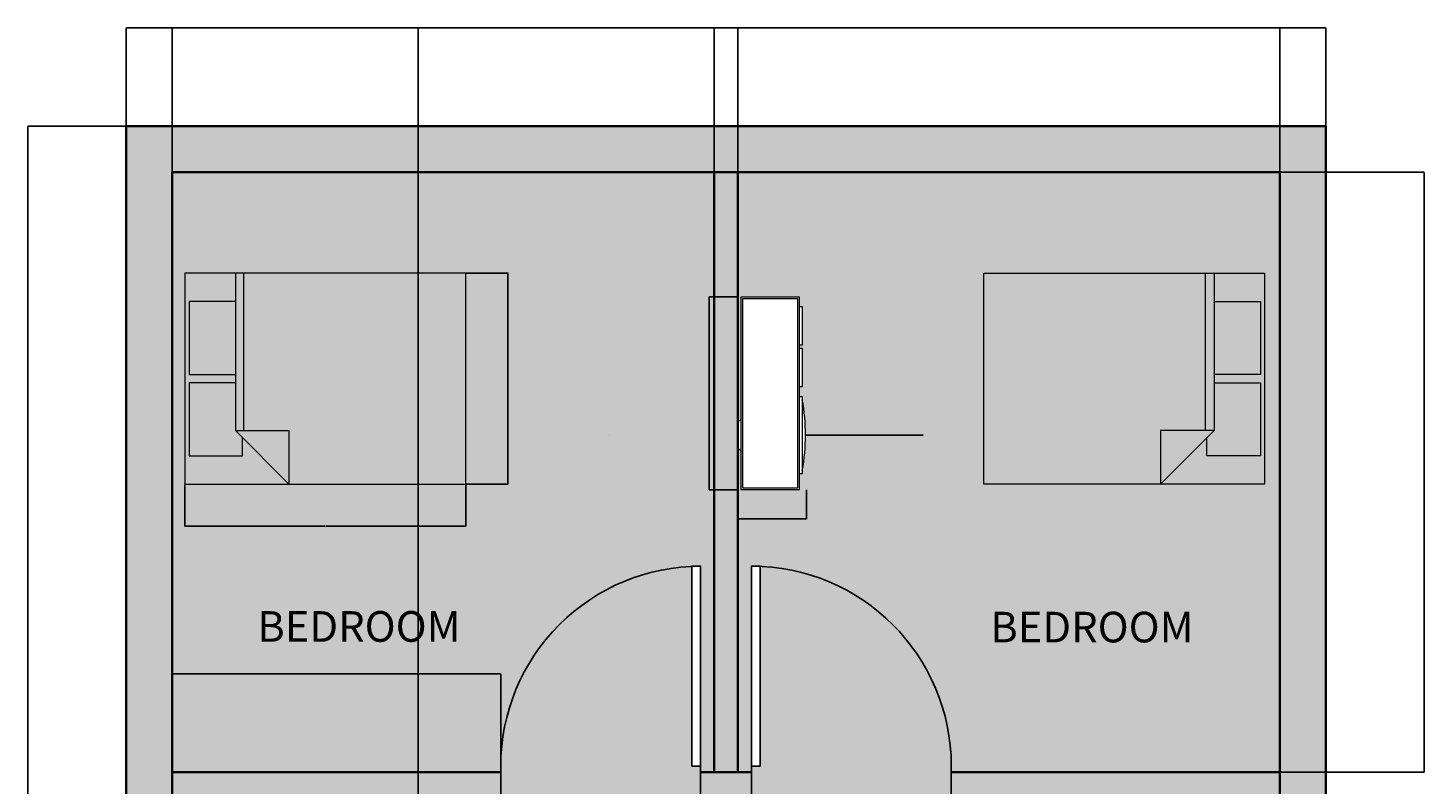
# Model space of a CAD drawing. Units: millimetres. Extents: x 1166 to 16630, y -7192 to 2820.
# Tile 8 of 8: x 9646 to 16630, y -963 to 2820. Entities that reach past the tile are written whole.
import ezdxf

# ---------------------------------------------------------------- set-up
doc = ezdxf.new("R2010")
doc.units = ezdxf.units.MM
for name, color, linetype, lineweight in [('A-ANNO-DIMS', 2, 'Continuous', 18), ('A-AREA-IDEN', 7, 'Continuous', 18), ('A-DOOR', 4, 'Continuous', 25), ('A-FURN', 8, 'Continuous', 18), ('A-WALL', 7, 'Continuous', 35)]:
    doc.layers.add(name, color=color, linetype=linetype, lineweight=lineweight)
for name, color, linetype, lineweight, true_color in [('A-FLOR-FNSH-PATT', 254, 'Continuous', 13, 0xfeeab9), ('A-FURN-PATT', 254, 'Continuous', 13, 0xd7c8d7), ('A-WALL-PATT', 254, 'Continuous', 13, 0xcecce6)]:
    doc.layers.add(name, color=color, linetype=linetype, lineweight=lineweight, true_color=true_color)
doc.styles.get("Standard").update_dxf_attribs({"font": 'arial.ttf'})
doc.dimstyles.get("Standard").update_dxf_attribs({"dimtxt": 0.18, "dimasz": 0.18, "dimexe": 0.18, "dimexo": 0.0625, "dimgap": 0.09, "dimtad": 0, "dimtih": 1, "dimtoh": 1, "dimdec": 4, "dimzin": 0, "dimdsep": 46, "dimtxsty": 'Standard', "dimcen": 0.09, "dimadec": 0, "dimazin": 0, "dimtfac": 1, "dimtdec": 4, "dimtofl": 0, "dimtmove": 0, "dimatfit": 3, "dimfxl": 1, "dimtolj": 1, "dimtzin": 0, "dimarcsym": 0})

# ---------------------------------------------------------------- blocks, each defined once
blk = doc.blocks.new('*U2')
for p, q in [((0, 0), (0, 6)), ((40, 0), (40, 6))]:
    blk.add_line(p, q)
blk.add_lwpolyline([(0, 0), (0, -40), (1.75, -40), (1.75, 0)], close=True)
blk.add_arc((0, 0), 40, 270, 0)
blk = doc.blocks.new('Bed - Queen')
for p, q in [((0, -80.00003), (0, 0)), ((0, 0), (59.99999, 0)), ((59.99999, 0), (59.99999, -80.00003)), ((7.99999, -1.2), (28.79998, -1.2)), ((7.99999, -14.4), (7.99999, -1.2)), ((28.79998, -1.2), (28.79998, -14.4)), ((31.19999, -1.2), (51.99999, -1.2)), ((31.19999, -14.4), (31.19999, -1.2)), ((51.99999, -1.2), (51.99999, -16.4)), ((0, -14.4), (44.8, -14.4)), ((59.99999, -29.6), (44.8, -14.4)), ((44.8, -14.4), (44.8, -29.6)), ((44.8, -16.8), (0, -16.8)), ((51.99999, -16.4), (46.79936, -16.4)), ((44.8, -29.6), (59.99999, -29.6)), ((59.99999, -80.00003), (0, -80.00003))]:
    blk.add_line(p, q)
blk = doc.blocks.new('Entertainment Center')
for p, q in [((-4, 0), (-5, -1)), ((4, 0), (-4, 0)), ((5, -1), (4, 0)), ((-17, -19), (-17, -1)), ((-17, -1), (43, -1)), ((-16.5, -18.5), (-16.5, -1.5)), ((-16.5, -1.5), (42.5, -1.5)), ((42.5, -1.5), (42.5, -18.5)), ((43, -1), (43, -19)), ((43, -19), (-17, -19)), ((42.5, -18.5), (-16.5, -18.5)), ((-12, -20), (-12, -19)), ((12, -20), (-12, -20)), ((12, -19), (12, -20)), ((15, -20), (15, -19)), ((27, -20), (15, -20)), ((27, -19), (27, -20)), ((28, -20), (28, -19)), ((40, -20), (28, -20)), ((40, -19), (40, -20))]:
    blk.add_line(p, q)
blk.add_arc((0, 40), 61, 259.6111, 280.3889)
blk = doc.blocks.new('*D15')
at = {"layer": 'A-ANNO-DIMS', "color": 0, "lineweight": -2, "transparency": 16777216}
for p, q in [((10431.5, 538.3), (10431.5, 327.4)), ((11836.7, 538.3), (11836.7, 327.4)), ((10431.7, 327.6), (11132.7, 327.6)), ((11836.6, 327.6), (11135.6, 327.6))]:
    blk.add_line(p, q, dxfattribs=at)
at = {"layer": 'A-ANNO-DIMS', "color": 0, "transparency": 16777216}
for points in [[(10431.7, 327.6), (10431.7, 327.5), (10431.5, 327.6)], [(11836.6, 327.6), (11836.6, 327.5), (11836.7, 327.6)]]:
    blk.add_solid(points, dxfattribs=at)
at = {"layer": 'Defpoints', "color": 0, "transparency": 16777216}
for p in [(10431.5, 538.4), (11836.7, 538.4), (10431.5, 327.6)]:
    blk.add_point(p, dxfattribs=at)
at = {"layer": 'A-ANNO-DIMS', "color": 0, "transparency": 16777216, "insert": (11134.1, 327.6), "char_height": 0.18, "attachment_point": 5}
blk.add_mtext('\\A1;QUEEN BED 1405 TYP.', dxfattribs=at)
blk = doc.blocks.new('*D16')
at = {"layer": 'A-ANNO-DIMS', "color": 0, "lineweight": -2, "transparency": 16777216}
for p, q in [((11836.8, 1592.3), (12047.7, 1592.3)), ((12047.5, 1592.1), (12047.5, 1065.5)), ((12047.5, 538.5), (12047.5, 1065.1)), ((11836.8, 538.4), (12047.7, 538.4))]:
    blk.add_line(p, q, dxfattribs=at)
at = {"layer": 'A-ANNO-DIMS', "color": 0, "transparency": 16777216}
for points in [[(12047.5, 1592.1), (12047.6, 1592.1), (12047.5, 1592.3)], [(12047.5, 538.5), (12047.6, 538.5), (12047.5, 538.4)]]:
    blk.add_solid(points, dxfattribs=at)
at = {"layer": 'Defpoints', "color": 0, "transparency": 16777216}
for p in [(11836.7, 1592.3), (11836.7, 538.4), (12047.5, 538.4)]:
    blk.add_point(p, dxfattribs=at)
at = {"layer": 'A-ANNO-DIMS', "color": 0, "transparency": 16777216, "insert": (12047.5, 1065.3), "char_height": 0.18, "attachment_point": 5}
blk.add_mtext('\\A1;1054 TYP.', dxfattribs=at)
blk = doc.blocks.new('*D19')
at = {"layer": 'A-ANNO-DIMS', "color": 0, "lineweight": -2, "transparency": 16777216}
for p, q in [((13198.1, 1474.7), (13053.2, 1474.7)), ((13053.4, 1474.5), (13053.4, 992.3)), ((13053.4, 509.7), (13053.4, 991.9)), ((13198.1, 509.5), (13053.2, 509.5))]:
    blk.add_line(p, q, dxfattribs=at)
at = {"layer": 'A-ANNO-DIMS', "color": 0, "transparency": 16777216}
for points in [[(13053.4, 1474.5), (13053.5, 1474.5), (13053.4, 1474.7)], [(13053.4, 509.7), (13053.5, 509.7), (13053.4, 509.5)]]:
    blk.add_solid(points, dxfattribs=at)
at = {"layer": 'Defpoints', "color": 0, "transparency": 16777216}
for p in [(13053.4, 1474.7), (13198.2, 1474.7), (13198.2, 509.5)]:
    blk.add_point(p, dxfattribs=at)
at = {"layer": 'A-ANNO-DIMS', "color": 0, "transparency": 16777216, "insert": (13053.4, 992.1), "char_height": 0.18, "attachment_point": 5}
blk.add_mtext('\\A1;TV UNIT 965', dxfattribs=at)
blk = doc.blocks.new('*D20')
at = {"layer": 'A-ANNO-DIMS', "color": 0, "lineweight": -2, "transparency": 16777216}
for p, q in [((13198.2, 509.5), (13198.2, 364.6)), ((13541.4, 509.5), (13541.4, 364.6)), ((13198.4, 364.7), (13369.5, 364.7)), ((13541.2, 364.7), (13370.1, 364.7))]:
    blk.add_line(p, q, dxfattribs=at)
at = {"layer": 'A-ANNO-DIMS', "color": 0, "transparency": 16777216}
for points in [[(13198.4, 364.8), (13198.4, 364.7), (13198.2, 364.7)], [(13541.2, 364.8), (13541.2, 364.7), (13541.4, 364.7)]]:
    blk.add_solid(points, dxfattribs=at)
at = {"layer": 'Defpoints', "color": 0, "transparency": 16777216}
for p in [(13198.2, 509.5), (13541.4, 509.5), (13198.2, 364.7)]:
    blk.add_point(p, dxfattribs=at)
at = {"layer": 'A-ANNO-DIMS', "color": 0, "transparency": 16777216, "insert": (13369.8, 364.7), "char_height": 0.18, "attachment_point": 5}
blk.add_mtext('\\A1;343', dxfattribs=at)
blk = doc.blocks.new('*D48')
at = {"layer": 'A-ANNO-DIMS', "color": 0, "lineweight": -2, "transparency": 16777216}
for p, q in [((10138.2, 2327.5), (10138.2, 2819.6)), ((10138.4, 2819.5), (13137.8, 2819.5)), ((16138, 2819.5), (13138.6, 2819.5)), ((16138.2, 2327.5), (16138.2, 2819.6))]:
    blk.add_line(p, q, dxfattribs=at)
at = {"layer": 'A-ANNO-DIMS', "color": 0, "transparency": 16777216}
for points in [[(10138.4, 2819.5), (10138.4, 2819.4), (10138.2, 2819.5)], [(16138, 2819.5), (16138, 2819.4), (16138.2, 2819.5)]]:
    blk.add_solid(points, dxfattribs=at)
at = {"layer": 'Defpoints', "color": 0, "transparency": 16777216}
for p in [(16138.2, 2819.5), (10138.2, 2327.5), (16138.2, 2327.5)]:
    blk.add_point(p, dxfattribs=at)
at = {"layer": 'A-ANNO-DIMS', "color": 0, "transparency": 16777216, "insert": (13138.2, 2819.5), "char_height": 0.18, "attachment_point": 5}
blk.add_mtext('\\A1;6000', dxfattribs=at)
blk = doc.blocks.new('*D49')
at = {"layer": 'A-ANNO-DIMS', "color": 0, "lineweight": -2, "transparency": 16777216}
for p, q in [((10138.1, 2327.5), (9646, 2327.5)), ((9646.2, 2327.3), (9646.2, -1676.3)), ((9646.2, -5680.2), (9646.2, -1676.6)), ((10138.1, -5680.3), (9646, -5680.3))]:
    blk.add_line(p, q, dxfattribs=at)
at = {"layer": 'A-ANNO-DIMS', "color": 0, "transparency": 16777216}
for points in [[(9646.2, 2327.3), (9646.2, 2327.3), (9646.2, 2327.5)], [(9646.2, -5680.2), (9646.2, -5680.2), (9646.2, -5680.3)]]:
    blk.add_solid(points, dxfattribs=at)
at = {"layer": 'Defpoints', "color": 0, "transparency": 16777216}
for p in [(10138.2, 2327.5), (9646.2, -5680.3), (10138.2, -5680.3)]:
    blk.add_point(p, dxfattribs=at)
at = {"layer": 'A-ANNO-DIMS', "color": 0, "transparency": 16777216, "insert": (9646.2, -1676.4), "char_height": 0.18, "attachment_point": 5}
blk.add_mtext('\\A1;8008', dxfattribs=at)
blk = doc.blocks.new('*D50')
at = {"layer": 'A-ANNO-DIMS', "color": 0, "lineweight": -2, "transparency": 16777216}
for p, q in [((10368.206606, 2097.524735), (10368.206606, 2819.642235)), ((10368.386606, 2819.462235), (11722.846606, 2819.462235)), ((13078.026606, 2819.462235), (11723.566606, 2819.462235)), ((13078.206606, 2097.524735), (13078.206606, 2819.642235))]:
    blk.add_line(p, q, dxfattribs=at)
at = {"layer": 'A-ANNO-DIMS', "color": 0, "transparency": 16777216}
for points in [[(10368.386606, 2819.492235), (10368.386606, 2819.432235), (10368.206606, 2819.462235)], [(13078.026606, 2819.492235), (13078.026606, 2819.432235), (13078.206606, 2819.462235)]]:
    blk.add_solid(points, dxfattribs=at)
at = {"layer": 'Defpoints', "color": 0, "transparency": 16777216}
for p in [(13078.206606, 2819.462235), (10368.206606, 2097.462235), (13078.206606, 2097.462235)]:
    blk.add_point(p, dxfattribs=at)
at = {"layer": 'A-ANNO-DIMS', "color": 0, "transparency": 16777216, "insert": (11723.206606, 2819.462235), "char_height": 0.18, "attachment_point": 5}
blk.add_mtext('\\A1;2710', dxfattribs=at)
blk = doc.blocks.new('*D51')
at = {"layer": 'A-ANNO-DIMS', "color": 0, "lineweight": -2, "transparency": 16777216}
for p, q in [((13198.206606, 2097.524735), (13198.206606, 2819.642235)), ((13198.386606, 2819.462235), (14552.846606, 2819.462235)), ((15908.026606, 2819.462235), (14553.566606, 2819.462235)), ((15908.206606, 2097.524735), (15908.206606, 2819.642235))]:
    blk.add_line(p, q, dxfattribs=at)
at = {"layer": 'A-ANNO-DIMS', "color": 0, "transparency": 16777216}
for points in [[(13198.386606, 2819.492235), (13198.386606, 2819.432235), (13198.206606, 2819.462235)], [(15908.026606, 2819.492235), (15908.026606, 2819.432235), (15908.206606, 2819.462235)]]:
    blk.add_solid(points, dxfattribs=at)
at = {"layer": 'Defpoints', "color": 0, "transparency": 16777216}
for p in [(15908.206606, 2819.462235), (13198.206606, 2097.462235), (15908.206606, 2097.462235)]:
    blk.add_point(p, dxfattribs=at)
at = {"layer": 'A-ANNO-DIMS', "color": 0, "transparency": 16777216, "insert": (14553.206606, 2819.462235), "char_height": 0.18, "attachment_point": 5}
blk.add_mtext('\\A1;2710', dxfattribs=at)
blk = doc.blocks.new('*D52')
at = {"layer": 'A-ANNO-DIMS', "color": 0, "lineweight": -2, "transparency": 16777216}
for p, q in [((15908.3, 2097.5), (16630.4, 2097.5)), ((16630.2, 2097.3), (16630.2, 597.6)), ((16630.2, -902.4), (16630.2, 597.3)), ((15908.3, -902.5), (16630.4, -902.5))]:
    blk.add_line(p, q, dxfattribs=at)
at = {"layer": 'A-ANNO-DIMS', "color": 0, "transparency": 16777216}
for points in [[(16630.2, 2097.3), (16630.2, 2097.3), (16630.2, 2097.5)], [(16630.2, -902.4), (16630.2, -902.4), (16630.2, -902.5)]]:
    blk.add_solid(points, dxfattribs=at)
at = {"layer": 'Defpoints', "color": 0, "transparency": 16777216}
for p in [(15908.2, 2097.5), (15908.2, -902.5), (16630.2, -902.5)]:
    blk.add_point(p, dxfattribs=at)
at = {"layer": 'A-ANNO-DIMS', "color": 0, "transparency": 16777216, "insert": (16630.2, 597.5), "char_height": 0.18, "attachment_point": 5}
blk.add_mtext('\\A1;3000', dxfattribs=at)
blk = doc.blocks.new('*D59')
at = {"layer": 'A-ANNO-DIMS', "color": 0, "lineweight": -2, "transparency": 16777216}
for p, q in [((12011.1, -902.6), (12011.1, -6172.5)), ((13011.1, -902.6), (13011.1, -6172.5)), ((12011.3, -6172.3), (12510.8, -6172.3)), ((13010.9, -6172.3), (12511.5, -6172.3))]:
    blk.add_line(p, q, dxfattribs=at)
at = {"layer": 'A-ANNO-DIMS', "color": 0, "transparency": 16777216}
for points in [[(12011.3, -6172.3), (12011.3, -6172.4), (12011.1, -6172.3)], [(13010.9, -6172.3), (13010.9, -6172.4), (13011.1, -6172.3)]]:
    blk.add_solid(points, dxfattribs=at)
at = {"layer": 'Defpoints', "color": 0, "transparency": 16777216}
for p in [(12011.1, -902.5), (13011.1, -902.5), (13011.1, -6172.3)]:
    blk.add_point(p, dxfattribs=at)
at = {"layer": 'A-ANNO-DIMS', "color": 0, "transparency": 16777216, "insert": (12511.1, -6172.3), "char_height": 0.18, "attachment_point": 5}
blk.add_mtext('\\A1;1000', dxfattribs=at)
blk = doc.blocks.new('*D60')
at = {"layer": 'A-ANNO-DIMS', "color": 0, "lineweight": -2, "transparency": 16777216}
for p, q in [((13265.3, -902.6), (13265.3, -6172.5)), ((14265.3, -902.6), (14265.3, -6172.5)), ((13265.5, -6172.3), (13765, -6172.3)), ((14265.1, -6172.3), (13765.7, -6172.3))]:
    blk.add_line(p, q, dxfattribs=at)
at = {"layer": 'A-ANNO-DIMS', "color": 0, "transparency": 16777216}
for points in [[(13265.5, -6172.3), (13265.5, -6172.4), (13265.3, -6172.3)], [(14265.1, -6172.3), (14265.1, -6172.4), (14265.3, -6172.3)]]:
    blk.add_solid(points, dxfattribs=at)
at = {"layer": 'Defpoints', "color": 0, "transparency": 16777216}
for p in [(13265.3, -902.5), (14265.3, -902.5), (14265.3, -6172.3)]:
    blk.add_point(p, dxfattribs=at)
at = {"layer": 'A-ANNO-DIMS', "color": 0, "transparency": 16777216, "insert": (13765.3, -6172.3), "char_height": 0.18, "attachment_point": 5}
blk.add_mtext('\\A1;1000', dxfattribs=at)
blk = doc.blocks.new('*D62')
at = {"layer": 'A-ANNO-DIMS', "color": 0, "lineweight": -2, "transparency": 16777216}
for p, q in [((10368.2, -4052.9), (10368.2, 2819.6)), ((10368.4, 2819.5), (10982.9, 2819.5)), ((11598.3, 2819.5), (10983.8, 2819.5)), ((11598.5, -4052.9), (11598.5, 2819.6))]:
    blk.add_line(p, q, dxfattribs=at)
at = {"layer": 'A-ANNO-DIMS', "color": 0, "transparency": 16777216}
for points in [[(10368.4, 2819.5), (10368.4, 2819.4), (10368.2, 2819.5)], [(11598.3, 2819.5), (11598.3, 2819.4), (11598.5, 2819.5)]]:
    blk.add_solid(points, dxfattribs=at)
at = {"layer": 'Defpoints', "color": 0, "transparency": 16777216}
for p in [(11598.5, 2819.5), (10368.2, -4053), (11598.5, -4053)]:
    blk.add_point(p, dxfattribs=at)
at = {"layer": 'A-ANNO-DIMS', "color": 0, "transparency": 16777216, "insert": (10983.4, 2819.5), "char_height": 0.18, "attachment_point": 5}
blk.add_mtext('\\A1;1230.3', dxfattribs=at)
blk = doc.blocks.new('*D65')
at = {"layer": 'A-ANNO-DIMS', "color": 0, "lineweight": -2, "transparency": 16777216}
for p, q in [((10368.2, -902.5), (10368.2, -410.4)), ((10368.4, -410.5), (11189.3, -410.5)), ((12010.9, -410.5), (11190, -410.5)), ((12011.1, -902.5), (12011.1, -410.4))]:
    blk.add_line(p, q, dxfattribs=at)
at = {"layer": 'A-ANNO-DIMS', "color": 0, "transparency": 16777216}
for points in [[(10368.4, -410.5), (10368.4, -410.6), (10368.2, -410.5)], [(12010.9, -410.5), (12010.9, -410.6), (12011.1, -410.5)]]:
    blk.add_solid(points, dxfattribs=at)
at = {"layer": 'Defpoints', "color": 0, "transparency": 16777216}
for p in [(12011.1, -410.5), (10368.2, -902.5), (12011.1, -902.5)]:
    blk.add_point(p, dxfattribs=at)
at = {"layer": 'A-ANNO-DIMS', "color": 0, "transparency": 16777216, "insert": (11189.7, -410.5), "char_height": 0.18, "attachment_point": 5}
blk.add_mtext('\\A1;1643', dxfattribs=at)
blk = doc.blocks.new('*D72')
at = {"layer": 'A-ANNO-DIMS', "color": 0, "lineweight": -2, "transparency": 16777216}
for p, q in [((12554.6, 783), (12554.8, 783)), ((12554.7, 782.9), (12554.7, 783.1)), ((14124.8, 783), (13536.2, 783))]:
    blk.add_line(p, q, dxfattribs=at)
at = {"layer": 'A-ANNO-DIMS', "color": 0, "transparency": 16777216}
blk.add_solid([(13536.2, 783), (13536.2, 783), (13536, 783)], dxfattribs=at)
at = {"layer": 'Defpoints', "color": 0, "transparency": 16777216}
for p in [(12554.7, 783), (13536, 783)]:
    blk.add_point(p, dxfattribs=at)
at = {"layer": 'A-ANNO-DIMS', "color": 0, "transparency": 16777216, "insert": (14125.3, 783), "char_height": 0.18, "attachment_point": 5}
blk.add_mtext('\\A1;R981.3', dxfattribs=at)

msp = doc.modelspace()

# ---------------------------------------------------------------- hatches: boundary and pattern name
at = {"layer": 'A-FLOR-FNSH-PATT', "transparency": 33554549}
h = msp.add_hatch(color=256, dxfattribs=at)
h.dxf.hatch_style = 1
h.paths.add_polyline_path([(14288.207, -1022.538), (14265.313, -1022.538), (14265.313, -872.538, 0.40145271), (13309.063, 126.505), (13309.063, -872.538), (13265.313, -872.538), (13265.313, -1022.538), (13011.1, -1022.538), (13011.1, -872.538), (12967.35, -872.538), (12967.35, 126.505, 0.40145271), (12011.1, -872.538), (12011.1, -1022.538), (11598.503, -1022.538), (11598.503, -1865.538), (11598.503, -3209.099), (11598.503, -4052.975), (13078.207, -4052.975), (13078.207, -3022.538), (14288.207, -3022.538), (14288.207, -2786.562), (14400.707, -2786.562), (14400.707, -2753.749), (15149.988, -2753.749, 0.40145271), (14400.707, -2036.562), (14288.207, -2036.562)])
h.paths.add_polyline_path([(11598.503, -1865.538), (11196.269, -1865.538), (11196.269, -3209.099), (11598.503, -3209.099)])
h.paths.add_polyline_path([(13078.207, 2097.462), (10368.207, 2097.462), (10368.207, -902.538), (12011.1, -902.538), (12011.1, -872.538, -0.40145271), (12967.35, 126.505), (12967.35, 127.462), (13011.1, 127.462), (13011.1, -872.538), (13011.1, -902.538), (13078.207, -902.538)])
h.paths.add_polyline_path([(11836.742, 538.355), (10431.54, 538.355), (10431.54, 1592.256), (11836.742, 1592.256)], flags=16)
h.paths.add_polyline_path([(10951.465, 538.355), (10719.606, 770.213), (10719.606, 678.875), (10452.618, 678.875), (10452.618, 1044.228), (10684.476, 1044.228), (10684.476, 1086.384), (10452.618, 1086.384), (10452.618, 1451.736), (10684.476, 1451.736), (10684.476, 805.343), (10951.465, 805.343)], flags=16)
h.paths.add_polyline_path([(15908.207, 2097.462), (13198.207, 2097.462), (13198.207, 847.342), (13214.293, 863.428), (13214.293, 1474.722), (13503.853, 1474.722), (13503.853, 1426.462), (13519.94, 1426.462), (13519.94, 1233.422), (13503.853, 1233.422), (13503.853, 1217.335), (13519.94, 1217.335), (13519.94, 1024.295), (13503.853, 1024.295), (13503.853, 976.035), (13519.94, 976.035), (13519.94, 959.948, -0.09090909), (13519.94, 606.042), (13519.94, 589.955), (13503.853, 589.955), (13503.853, 509.522), (13214.293, 509.522), (13214.293, 702.562), (13198.207, 718.648), (13198.207, -902.538), (13265.313, -902.538), (13265.313, -872.538), (13265.313, 127.462), (13309.063, 127.462), (13309.063, 126.505, -0.40145271), (14265.313, -872.538), (14265.313, -902.538), (15908.207, -902.538)])
h.paths.add_polyline_path([(14427.327, 538.355), (14427.327, 1592.256), (15832.53, 1592.256), (15832.53, 538.355)], flags=16)
h.paths.add_polyline_path([(15312.605, 538.355), (15312.605, 805.343), (15579.593, 805.343), (15579.593, 1451.736), (15811.452, 1451.736), (15811.452, 1086.384), (15579.593, 1086.384), (15579.593, 1044.228), (15811.452, 1044.228), (15811.452, 678.875), (15544.463, 678.875), (15544.463, 770.213)], flags=16)
h.paths.add_polyline_path([(12516.729, -2244.054), (13499.854, -2244.054), (13499.854, -2006.254), (12516.729, -2006.254)], flags=24)
h.paths.add_polyline_path([(11791.983, -3737.781), (12263.574, -3737.781), (12263.574, -3444.03), (11791.983, -3444.03)], flags=24)
h.paths.add_polyline_path([(10753.982, -293.014), (11939.114, -293.014), (11939.114, -55.214), (10753.982, -55.214)], flags=24)
h.paths.add_polyline_path([(14420.893, -296.216), (15606.026, -296.216), (15606.026, -58.416), (14420.893, -58.416)], flags=24)
at = {"layer": 'A-FURN-PATT'}
h = msp.add_hatch(color=256, dxfattribs=at)
h.dxf.hatch_style = 1
h.paths.add_polyline_path([(15832.53, 1592.256), (15579.593, 1592.256), (15579.593, 1451.736), (15811.452, 1451.736), (15811.452, 1086.384), (15579.593, 1086.384), (15579.593, 1044.228), (15811.452, 1044.228), (15811.452, 678.875), (15544.463, 678.875), (15544.463, 770.213), (15312.605, 538.355), (15832.53, 538.355)])
h.paths.add_polyline_path([(15579.593, 1592.256), (15537.437, 1592.256), (15537.437, 805.343), (15579.593, 805.343)], flags=17)
h.paths.add_polyline_path([(10684.476, 1592.256), (10431.54, 1592.256), (10431.54, 538.355), (10951.465, 538.355), (10719.606, 770.213), (10719.606, 678.875), (10452.618, 678.875), (10452.618, 1044.228), (10684.476, 1044.228), (10684.476, 1086.384), (10452.618, 1086.384), (10452.618, 1451.736), (10684.476, 1451.736)])
h.paths.add_polyline_path([(10726.632, 1592.256), (10684.476, 1592.256), (10684.476, 805.343), (10726.632, 805.343)], flags=17)
h.paths.add_polyline_path([(10951.465, 805.343), (10684.476, 805.343), (10951.465, 538.355)])
h = msp.add_hatch(color=256, dxfattribs=at)
h.dxf.hatch_style = 1
h.paths.add_polyline_path([(15537.437, 1592.256), (14427.327, 1592.256), (14427.327, 538.355), (15312.605, 538.355), (15312.605, 805.343), (15537.437, 805.343)])
h.paths.add_polyline_path([(11836.742, 1592.256), (10726.632, 1592.256), (10726.632, 805.343), (10951.465, 805.343), (10951.465, 538.355), (11836.742, 538.355)])
h = msp.add_hatch(color=256, dxfattribs=at)
h.dxf.hatch_style = 1
h.paths.add_polyline_path([(10684.476, 1451.736), (10452.618, 1451.736), (10452.618, 1086.384), (10684.476, 1086.384)])
h.paths.add_polyline_path([(10684.476, 1044.228), (10452.618, 1044.228), (10452.618, 678.875), (10719.606, 678.875), (10719.606, 770.213), (10684.476, 805.343)])
h.paths.add_polyline_path([(15579.593, 805.343), (15312.605, 805.343), (15312.605, 538.355)])
h.paths.add_polyline_path([(15811.452, 1451.736), (15579.593, 1451.736), (15579.593, 1086.384), (15811.452, 1086.384)])
h.paths.add_polyline_path([(15811.452, 1044.228), (15579.593, 1044.228), (15579.593, 805.343), (15544.463, 770.213), (15544.463, 678.875), (15811.452, 678.875)])
at = {"layer": 'A-WALL-PATT'}
h = msp.add_hatch(color=256, dxfattribs=at)
h.dxf.hatch_style = 1
h.paths.add_polyline_path([(10138.207, 2327.462), (10138.207, -5680.344), (16138.207, -5680.344), (16138.207, 2327.462)])
h.paths.add_polyline_path([(15908.207, 2097.462), (15908.207, -5450.344), (10368.207, -5450.344), (10368.207, 2097.462)], flags=16)
h.paths.add_polyline_path([(14427.327, 1592.256), (15832.53, 1592.256), (15832.53, 538.355), (14427.327, 538.355)], flags=0)
h.paths.add_polyline_path([(15579.593, 805.343), (15579.593, 1451.736), (15811.452, 1451.736), (15811.452, 1086.384), (15579.593, 1086.384), (15579.593, 1044.228), (15811.452, 1044.228), (15811.452, 678.875), (15544.463, 678.875), (15544.463, 770.213), (15312.605, 538.355), (15312.605, 805.343)], flags=0)
h.paths.add_polyline_path([(11598.503, -1022.538), (11598.503, -1865.538), (11598.503, -3209.099), (11598.503, -4052.099), (11598.503, -4052.975), (10368.207, -4052.975), (10784.05, -3631.037), (10704.756, -3631.037), (10704.756, -1444.038), (10782.238, -1444.038), (10368.207, -1022.538)], flags=0)
h.paths.add_polyline_path([(12967.35, 127.462), (13011.1, 127.462), (13011.1, -872.538), (12967.35, -872.538)], flags=0)
h.paths.add_polyline_path([(12712.811, -4827.516), (13814.967, -4827.516), (13814.967, -4589.717), (12712.811, -4589.717)], flags=8)
h.paths.add_polyline_path([(12516.729, -2244.054), (13499.854, -2244.054), (13499.854, -2006.254), (12516.729, -2006.254)], flags=8)
h.paths.add_polyline_path([(14678.782, -1737.829), (15507.241, -1737.829), (15507.241, -1500.03), (14678.782, -1500.03)], flags=8)
h.paths.add_polyline_path([(14420.893, -296.216), (15606.026, -296.216), (15606.026, -58.416), (14420.893, -58.416)], flags=8)
h.paths.add_polyline_path([(10753.982, -293.014), (11939.114, -293.014), (11939.114, -55.214), (10753.982, -55.214)], flags=8)
h.paths.add_polyline_path([(11791.983, -3737.781), (12263.574, -3737.781), (12263.574, -3444.03), (11791.983, -3444.03)], flags=8)
h = msp.add_hatch(color=256, dxfattribs=at)
h.dxf.hatch_style = 1
h.paths.add_polyline_path([(13198.207, -3142.538), (14288.207, -3142.538), (15908.207, -3142.538), (15908.207, -3022.538), (14408.207, -3022.538), (14408.207, -2786.562), (14400.707, -2786.562), (14288.207, -2786.562), (14288.207, -3022.538), (13078.207, -3022.538), (13078.207, -4052.975), (10368.207, -4052.975), (10368.207, -4282.975), (13198.207, -4282.975)])
h.paths.add_polyline_path([(12011.1, -902.538), (10368.207, -902.538), (10368.207, -1022.538), (12011.1, -1022.538)])
h.paths.add_polyline_path([(13198.207, 2097.462), (13078.207, 2097.462), (13078.207, -902.538), (13198.207, -902.538)])
h.paths.add_polyline_path([(15908.207, -902.538), (14265.313, -902.538), (14265.313, -1022.538), (15908.207, -1022.538)])
h.paths.add_polyline_path([(14408.207, -1022.538), (14288.207, -1022.538), (14288.207, -2036.562), (14408.207, -2036.562)])
h.paths.add_polyline_path([(13265.313, -902.538), (13011.1, -902.538), (13011.1, -1022.538), (13265.313, -1022.538)])

# ---------------------------------------------------------------- linework, layer by layer
at = {"layer": 'A-WALL'}
for p, q in [((10138.207, 2327.462), (16138.207, 2327.462)), ((10138.207, -5680.344), (10138.207, 2327.462)), ((16138.207, 2327.462), (16138.207, -5680.344)), ((10368.207, 2097.462), (15908.207, 2097.462)), ((10368.207, -5450.344), (10368.207, 2097.462)), ((13078.207, 2097.462), (13078.207, -902.538)), ((13198.207, 2097.462), (13198.207, -902.538)), ((15908.207, 2097.462), (15908.207, -5450.344)), ((10368.207, -902.538), (12011.1, -902.538)), ((13011.1, -902.538), (13265.313, -902.538)), ((14265.313, -902.538), (15908.207, -902.538))]:
    msp.add_line(p, q, dxfattribs=at)

# ---------------------------------------------------------------- block references
at = {"layer": 'A-DOOR', "yscale": 25, "zscale": 25, "rotation": 180}
for p, xscale in [((13011.1, -872.538), 25), ((13265.313, -872.538), -25)]:
    msp.add_blockref('*U2', p, dxfattribs=dict(at, xscale=xscale))
at = {"layer": 'A-FURN'}
for name, p, xscale, yscale, zscale, rotation in [('Bed - Queen', (10431.54, 1592.256), -17.56502283482635, 17.56502283482635, 17.56502283482635, 90), ('Bed - Queen', (15832.53, 1592.256), 17.56502283482635, 17.56502283482635, 17.56502283482635, 270), ('Entertainment Center', (13198.207, 782.995), 16.08666666666661, 16.08666666666661, 16.08666666666661, 90)]:
    msp.add_blockref(name, p, dxfattribs=dict(at, xscale=xscale, yscale=yscale, zscale=zscale, rotation=rotation))

# ---------------------------------------------------------------- texts
at = {"layer": 'A-AREA-IDEN'}
for p in [(10793.615, -250.768), (14460.527, -253.97)]:
    msp.add_text('BEDROOM', height=153.2035, dxfattribs=at).set_placement(p)

# ---------------------------------------------------------------- dimensions: what is measured, and where the dimension line sits
at = {"layer": 'A-ANNO-DIMS'}
for base, p1, p2, override, picture, middle in [((16138.207, 2819.462), (10138.207, 2327.462), (16138.207, 2327.462), {"dimdec": 0, "dimlfac": 1, "dimrnd": 0, "dimzin": 0, "dimdsep": 46, "dimlunit": 2}, '*D48', (13138.207, 2819.462)), ((13078.207, 2819.462), (10368.207, 2097.462), (13078.207, 2097.462), {"dimdec": 0, "dimlfac": 1, "dimrnd": 0, "dimzin": 0, "dimdsep": 46, "dimlunit": 2}, '*D50', (11723.207, 2819.462)), ((11598.503, 2819.462), (10368.207, -4052.975), (11598.503, -4052.975), {"dimdec": 1, "dimlfac": 1, "dimrnd": 0, "dimzin": 0, "dimdsep": 46, "dimlunit": 2}, '*D62', (10983.355, 2819.462)), ((15908.207, 2819.462), (13198.207, 2097.462), (15908.207, 2097.462), {"dimdec": 0, "dimlfac": 1, "dimrnd": 0, "dimzin": 0, "dimdsep": 46, "dimlunit": 2}, '*D51', (14553.207, 2819.462)), ((12011.1, -410.538), (10368.207, -902.538), (12011.1, -902.538), {"dimdec": 0, "dimlfac": 1, "dimrnd": 0, "dimzin": 0, "dimdsep": 46, "dimlunit": 2}, '*D65', (11189.654, -410.538)), ((13011.1, -6172.344), (12011.1, -902.538), (13011.1, -902.538), {"dimdec": 0, "dimlfac": 1, "dimrnd": 0, "dimzin": 0, "dimdsep": 46, "dimlunit": 2}, '*D59', (12511.1, -6172.344)), ((14265.313, -6172.344), (13265.313, -902.538), (14265.313, -902.538), {"dimdec": 0, "dimlfac": 1, "dimrnd": 0, "dimzin": 0, "dimdsep": 46, "dimlunit": 2}, '*D60', (13765.313, -6172.344))]:
    dim = msp.add_linear_dim(base=base, p1=p1, p2=p2, dimstyle='Standard', override=override, dxfattribs=at)
    dim.commit()
    dim.dimension.update_dxf_attribs({"geometry": picture, "text_midpoint": middle})
for base, p1, p2, angle, picture, middle in [((9646.207, -5680.344), (10138.207, 2327.462), (10138.207, -5680.344), 90, '*D49', (9646.207, -1676.441)), ((16630.207, -902.538), (15908.207, 2097.462), (15908.207, -902.538), 90, '*D52', (16630.207, 597.462)), ((13198.207, 364.742), (13541.389, 509.522), (13198.207, 509.522), 180, '*D20', (13369.798, 364.742))]:
    dim = msp.add_linear_dim(base=base, p1=p1, p2=p2, angle=angle, dimstyle='Standard', override={"dimdec": 0, "dimlfac": 1, "dimrnd": 0, "dimzin": 0, "dimdsep": 46, "dimlunit": 2}, dxfattribs=at)
    dim.commit()
    dim.dimension.update_dxf_attribs({"geometry": picture, "text_midpoint": middle})
for base, p1, p2, angle, text, picture, middle in [((12047.523, 538.355), (11836.742, 1592.256), (11836.742, 538.355), 270, '<> TYP.', '*D16', (12047.523, 1065.305)), ((13053.427, 1474.722), (13198.207, 509.522), (13198.207, 1474.722), 90, 'TV UNIT <>', '*D19', (13053.427, 992.122)), ((10431.54, 327.575), (11836.742, 538.355), (10431.54, 538.355), 180, 'QUEEN BED <> TYP.', '*D15', (11134.141, 327.575))]:
    dim = msp.add_linear_dim(base=base, p1=p1, p2=p2, angle=angle, text=text, dimstyle='Standard', override={"dimdec": 0, "dimlfac": 1, "dimrnd": 0, "dimzin": 0, "dimdsep": 46, "dimlunit": 2}, dxfattribs=at)
    dim.commit()
    dim.dimension.update_dxf_attribs({"geometry": picture, "text_midpoint": middle})
dim = msp.add_radius_dim(center=(12554.74, 782.995), mpoint=(13536.027, 782.995), dimstyle='Standard', override={"dimdec": 1, "dimlfac": 1, "dimrnd": 0, "dimzin": 0, "dimdsep": 46, "dimlunit": 2}, dxfattribs=at)
dim.commit()
dim.dimension.update_dxf_attribs({"geometry": '*D72', "text_midpoint": (14124.799, 782.995), "dimtype": 164})

doc.saveas('drawing.dxf')
